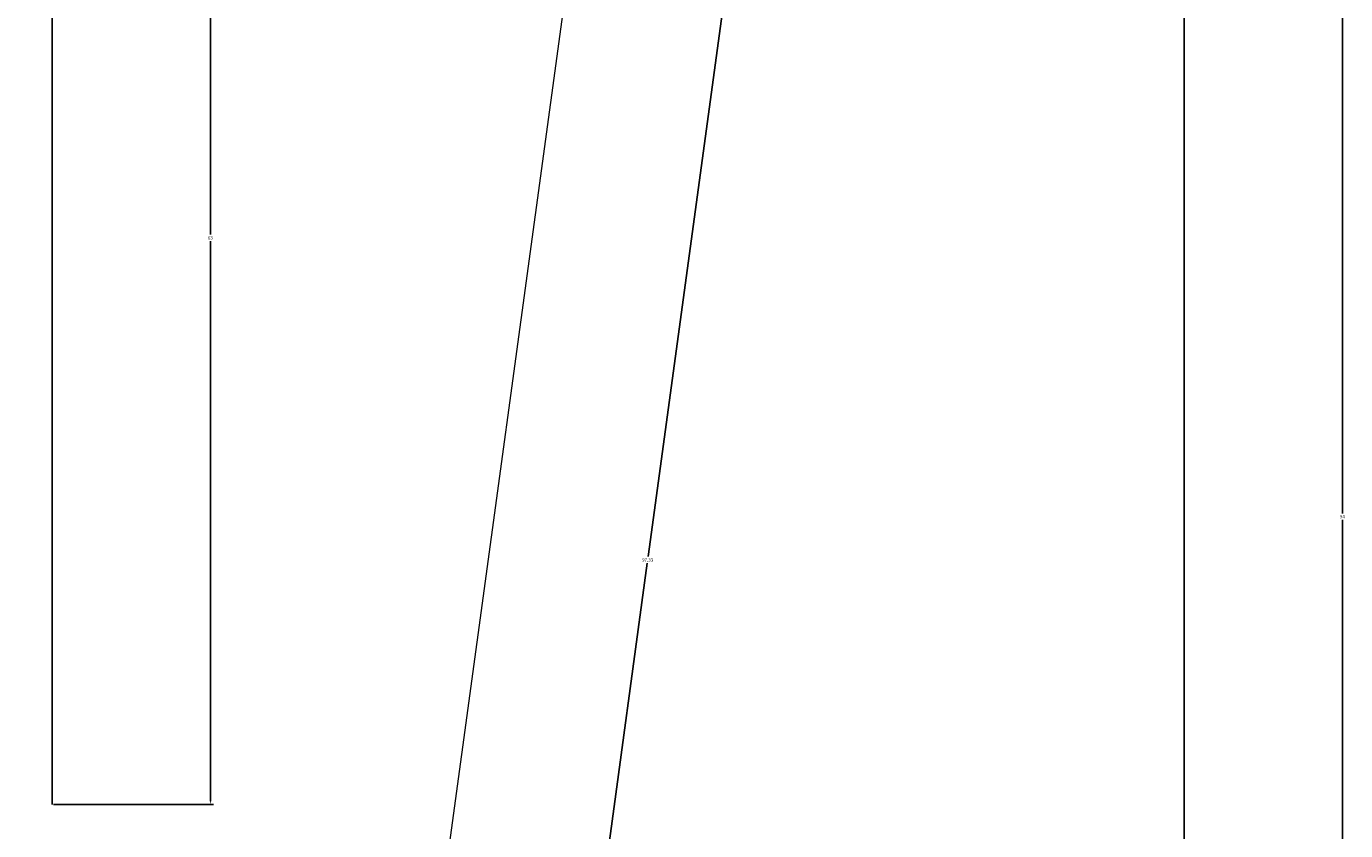
# Model space of a CAD drawing. Units: millimetres. Extents: x -9 to 135, y -119 to 27.
# Tile 6 of 12: x 62 to 135, y -63 to -18. Entities that reach past the tile are written whole.
import ezdxf

# ---------------------------------------------------------------- set-up
doc = ezdxf.new("R2010")
doc.units = ezdxf.units.MM
doc.layers.add('M-CONS', color=8, linetype='Continuous', lineweight=18)
doc.layers.add('M-DIMS', color=2, linetype='Continuous', lineweight=18)
doc.styles.get("Standard").update_dxf_attribs({"font": 'arial.ttf'})
doc.dimstyles.get("Standard").update_dxf_attribs({"dimtxt": 0.18, "dimasz": 0.18, "dimexe": 0.18, "dimexo": 0.0625, "dimgap": 0.09, "dimtad": 0, "dimtih": 1, "dimtoh": 1, "dimdec": 4, "dimzin": 0, "dimdsep": 46, "dimtxsty": 'Standard', "dimcen": 0.09, "dimadec": 0, "dimazin": 0, "dimtfac": 1, "dimtdec": 4, "dimtofl": 0, "dimtmove": 0, "dimatfit": 3, "dimfxl": 1, "dimtolj": 1, "dimtzin": 0, "dimarcsym": 0})

# ---------------------------------------------------------------- blocks, each defined once
blk = doc.blocks.new('*D3')
at = {"layer": 'Defpoints', "color": 0, "transparency": 16777216}
for p in [(0, 17.733), (-8.8, -110.267), (63, -110.267)]:
    blk.add_point(p, dxfattribs=at)
at = {"layer": 'M-DIMS', "color": 0, "lineweight": -2, "transparency": 16777216}
for p, q in [((-0.062, 17.733), (-8.98, 17.733)), ((-8.8, 17.553), (-8.8, -46.085)), ((-8.8, -110.087), (-8.8, -46.449)), ((62.938, -110.267), (-8.98, -110.267))]:
    blk.add_line(p, q, dxfattribs=at)
at = {"layer": 'M-DIMS', "color": 0, "transparency": 16777216}
for points in [[(-8.83, 17.553), (-8.77, 17.553), (-8.8, 17.733)], [(-8.83, -110.087), (-8.77, -110.087), (-8.8, -110.267)]]:
    blk.add_solid(points, dxfattribs=at)
at = {"layer": 'M-DIMS', "color": 0, "transparency": 16777216, "insert": (-8.8, -46.267), "char_height": 0.18, "attachment_point": 5}
blk.add_mtext('\\A1;128', dxfattribs=at)
blk = doc.blocks.new('*D12')
at = {"layer": 'Defpoints', "color": 0, "transparency": 16777216}
for p in [(63, 1.733), (63, -61.267), (71.8, -61.267)]:
    blk.add_point(p, dxfattribs=at)
at = {"layer": 'M-DIMS', "color": 0, "lineweight": -2, "transparency": 16777216}
for p, q in [((63.063, 1.733), (71.98, 1.733)), ((71.8, 1.553), (71.8, -29.585)), ((71.8, -61.087), (71.8, -29.949)), ((63.063, -61.267), (71.98, -61.267))]:
    blk.add_line(p, q, dxfattribs=at)
at = {"layer": 'M-DIMS', "color": 0, "transparency": 16777216}
for points in [[(71.77, 1.553), (71.83, 1.553), (71.8, 1.733)], [(71.77, -61.087), (71.83, -61.087), (71.8, -61.267)]]:
    blk.add_solid(points, dxfattribs=at)
at = {"layer": 'M-DIMS', "color": 0, "transparency": 16777216, "insert": (71.8, -29.767), "char_height": 0.18, "attachment_point": 5}
blk.add_mtext('\\A1;63', dxfattribs=at)
blk = doc.blocks.new('*D13')
at = {"layer": 'Defpoints', "color": 0, "transparency": 16777216}
for p in [(126, 1.733), (63, -92.267), (134.8, -92.267)]:
    blk.add_point(p, dxfattribs=at)
at = {"layer": 'M-DIMS', "color": 0, "lineweight": -2, "transparency": 16777216}
for p, q in [((126.062, 1.733), (134.98, 1.733)), ((134.8, 1.553), (134.8, -45.085)), ((134.8, -92.087), (134.8, -45.449)), ((63.063, -92.267), (134.98, -92.267))]:
    blk.add_line(p, q, dxfattribs=at)
at = {"layer": 'M-DIMS', "color": 0, "transparency": 16777216}
for points in [[(134.77, 1.553), (134.83, 1.553), (134.8, 1.733)], [(134.77, -92.087), (134.83, -92.087), (134.8, -92.267)]]:
    blk.add_solid(points, dxfattribs=at)
at = {"layer": 'M-DIMS', "color": 0, "transparency": 16777216, "insert": (134.8, -45.267), "char_height": 0.18, "attachment_point": 5}
blk.add_mtext('\\A1;94', dxfattribs=at)
blk = doc.blocks.new('*D15')
at = {"layer": 'Defpoints', "color": 0, "transparency": 16777216}
for p in [(94, 1.733), (80.835, -94.702), (89.554, -95.892)]:
    blk.add_point(p, dxfattribs=at)
at = {"layer": 'M-DIMS', "color": 0, "lineweight": -2, "transparency": 16777216}
for p, q in [((94.062, 1.725), (102.897, 0.519)), ((102.695, 0.365), (96.161, -47.493)), ((89.578, -95.714), (96.112, -47.856)), ((80.896, -94.71), (89.732, -95.916))]:
    blk.add_line(p, q, dxfattribs=at)
at = {"layer": 'M-DIMS', "color": 0, "transparency": 16777216}
for points in [[(102.665, 0.369), (102.724, 0.36), (102.719, 0.543)], [(89.548, -95.71), (89.608, -95.718), (89.554, -95.892)]]:
    blk.add_solid(points, dxfattribs=at)
at = {"layer": 'M-DIMS', "color": 0, "transparency": 16777216, "insert": (96.136, -47.675), "char_height": 0.18, "attachment_point": 5}
blk.add_mtext('\\A1;97.33', dxfattribs=at)
blk = doc.blocks.new('*D16')
at = {"layer": 'Defpoints', "color": 0, "transparency": 16777216}
for p in [(126, 1.733), (63, -92.267), (126, -119.067)]:
    blk.add_point(p, dxfattribs=at)
at = {"layer": 'M-DIMS', "color": 0, "lineweight": -2, "transparency": 16777216}
for p, q in [((126, 1.671), (126, -119.247)), ((63, -92.329), (63, -119.247)), ((63.18, -119.067), (94.281, -119.067)), ((125.82, -119.067), (94.719, -119.067))]:
    blk.add_line(p, q, dxfattribs=at)
at = {"layer": 'M-DIMS', "color": 0, "transparency": 16777216}
for points in [[(63.18, -119.037), (63.18, -119.097), (63, -119.067)], [(125.82, -119.037), (125.82, -119.097), (126, -119.067)]]:
    blk.add_solid(points, dxfattribs=at)
at = {"layer": 'M-DIMS', "color": 0, "transparency": 16777216, "insert": (94.5, -119.067), "char_height": 0.18, "attachment_point": 5}
blk.add_mtext('\\A1;63', dxfattribs=at)

msp = doc.modelspace()

# ---------------------------------------------------------------- linework, layer by layer
at = {"layer": 'M-CONS'}
msp.add_line((94, 1.733, 115.129), (80.835, -94.702, 115.129), dxfattribs=at)
msp.add_polyline3d([(63, 1.733, 115.129), (63, -61.267, 115.129), (63, 1.733, 71.129)], close=True, dxfattribs=at)

# ---------------------------------------------------------------- dimensions: what is measured, and where the dimension line sits
at = {"layer": 'M-DIMS'}
for base, p1, p2, angle, override, picture, middle in [((-8.8, -110.267), (0, 17.733), (63, -110.267), 90, {"dimdec": 0, "dimlfac": 1, "dimrnd": 0, "dimzin": 0, "dimdsep": 46, "dimlunit": 2}, '*D3', (-8.8, -46.267)), ((71.8, -61.267), (63, 1.733), (63, -61.267), 270, {"dimdec": 0, "dimlfac": 1, "dimrnd": 0, "dimzin": 0, "dimdsep": 46, "dimlunit": 2}, '*D12', (71.8, -29.767)), ((134.8, -92.267), (126, 1.733), (63, -92.267), 90, {"dimdec": 0, "dimlfac": 1, "dimrnd": 0, "dimzin": 0, "dimdsep": 46, "dimlunit": 2}, '*D13', (134.8, -45.267)), ((89.554, -95.892), (94, 1.733), (80.835, -94.702), 262.22595, {"dimdec": 2, "dimlfac": 1, "dimrnd": 0, "dimzin": 0, "dimdsep": 46, "dimlunit": 2}, '*D15', (96.136, -47.675))]:
    dim = msp.add_linear_dim(base=base, p1=p1, p2=p2, angle=angle, dimstyle='Standard', override=override, dxfattribs=at)
    dim.commit()
    dim.dimension.update_dxf_attribs({"geometry": picture, "text_midpoint": middle})
dim = msp.add_linear_dim(base=(126, -119.067), p1=(63, -92.267), p2=(126, 1.733), dimstyle='Standard', override={"dimdec": 0, "dimlfac": 1, "dimrnd": 0, "dimzin": 0, "dimdsep": 46, "dimlunit": 2}, dxfattribs=at)
dim.commit()
dim.dimension.update_dxf_attribs({"geometry": '*D16', "text_midpoint": (94.5, -119.067)})

doc.saveas('drawing.dxf')
